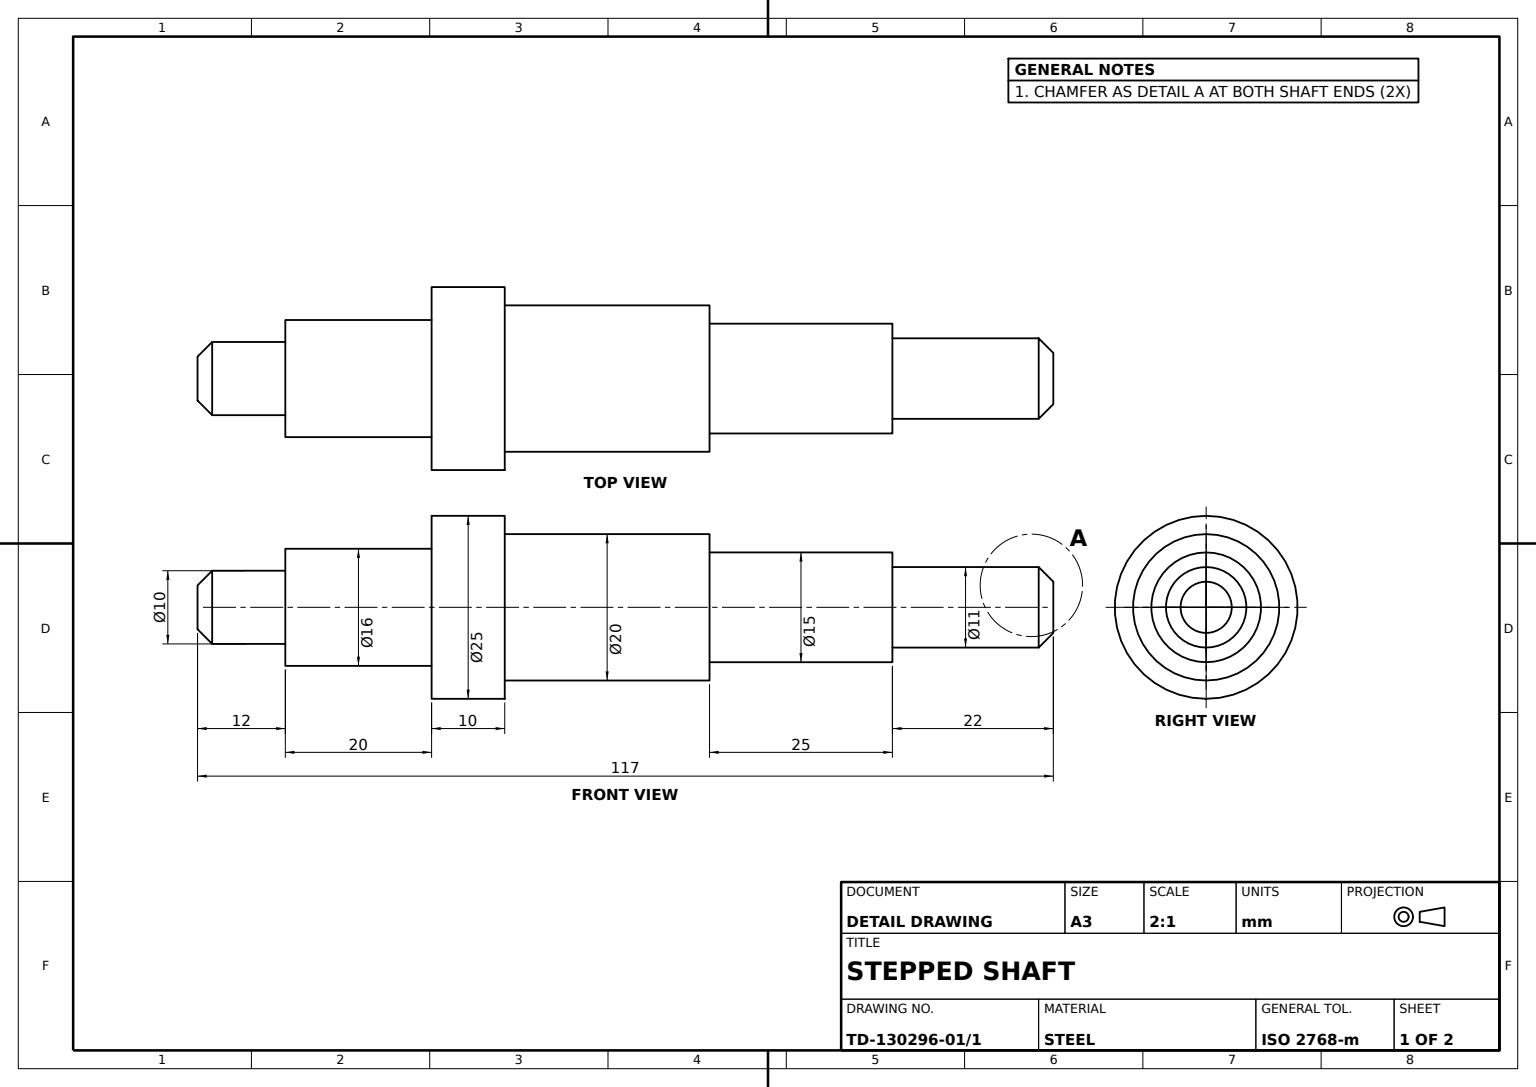
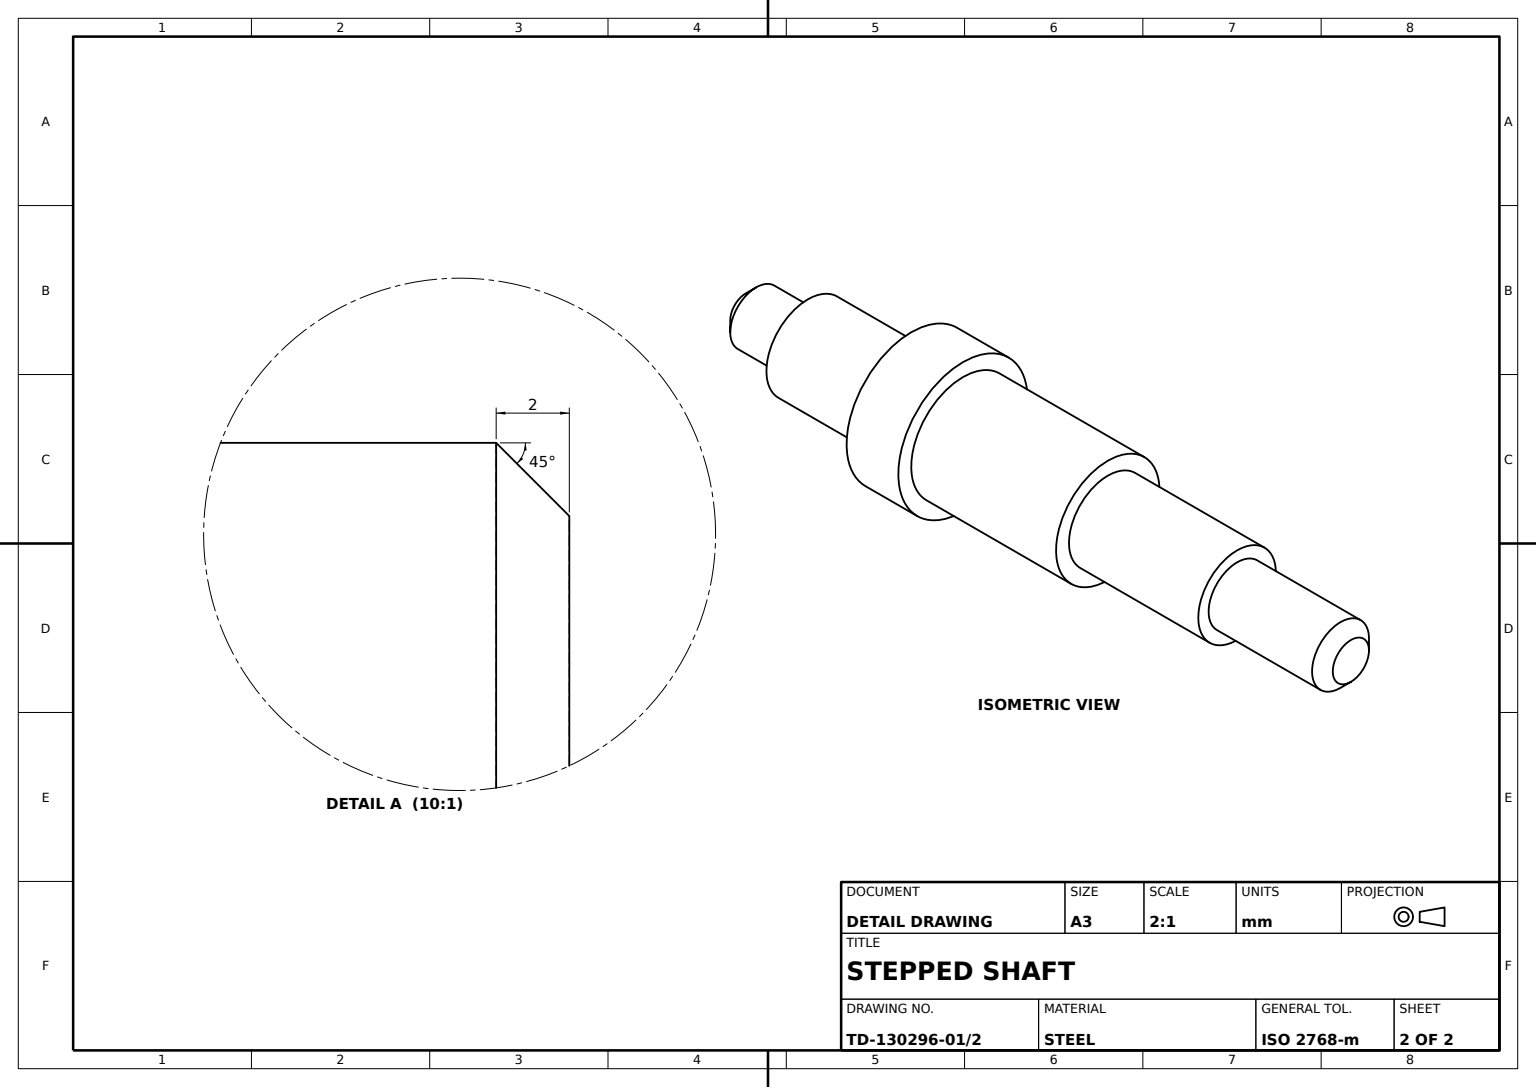
SolidWorks part; units mm, degrees
material "Plain Carbon Steel"
ref_plane "Front Plane" through (0, 0, 0) normal (0, 0, 1) x (1, 0, 0)
ref_plane "Top Plane" through (0, 0, 0) normal (0, 1, 0) x (1, 0, 0)
ref_plane "Right Plane" through (0, 0, 0) normal (1, 0, 0) x (0, 0, -1)
sketch "Shaft Profile Sketch" plane through (0, 0, 0) normal (0, 0, 1) x (1, 0, 0)
  line L0 (-58.5, 0) -> (58.5, 0) construction
  line L1 (-58.5, 0) -> (-58.5, -5)
  line L2 (-58.5, -5) -> (-46.5, -5)
  line L3 (-46.5, -5) -> (-46.5, -8)
  line L4 (-46.5, -8) -> (-26.5, -8)
  line L5 (-26.5, -8) -> (-26.5, -12.5)
  line L6 (-26.5, -12.5) -> (-16.5, -12.5)
  line L7 (-16.5, -12.5) -> (-16.5, -10)
  line L8 (-16.5, -10) -> (11.5, -10)
  line L9 (11.5, -10) -> (11.5, -7.5)
  line L10 (11.5, -7.5) -> (36.5, -7.5)
  line L11 (36.5, -7.5) -> (36.5, -5.5)
  line L12 (36.5, -5.5) -> (58.5, -5.5)
  line L13 (58.5, -5.5) -> (58.5, 0)
  line L14 (-58.5, 0) -> (58.5, 0) construction
  line L15 (-58.5, 0) -> (58.5, 0) construction
  line L16 (-58.5, 0) -> (58.5, 0)
  point P11 (0, 0)
  dimension "D1" = 117
  dimension "D2" = 12
  dimension "D3" = 22
  dimension "D4" = 25
  dimension "D5" = 28
  dimension "D6" = 10
  dimension "D7" = 10
  dimension "D8" = 16
  dimension "D9" = 25
  dimension "D10" = 20
  dimension "D11" = 15
  dimension "D12" = 11
revolve "Stepped Shaft Revolve" add sketch "Shaft Profile Sketch" angle 360 about L0
chamfer "Edge Chamfer 2x45°" distance 2 angle 45 2 edges at (-58.5, -5, 0) (58.5, -5.5, 0)
